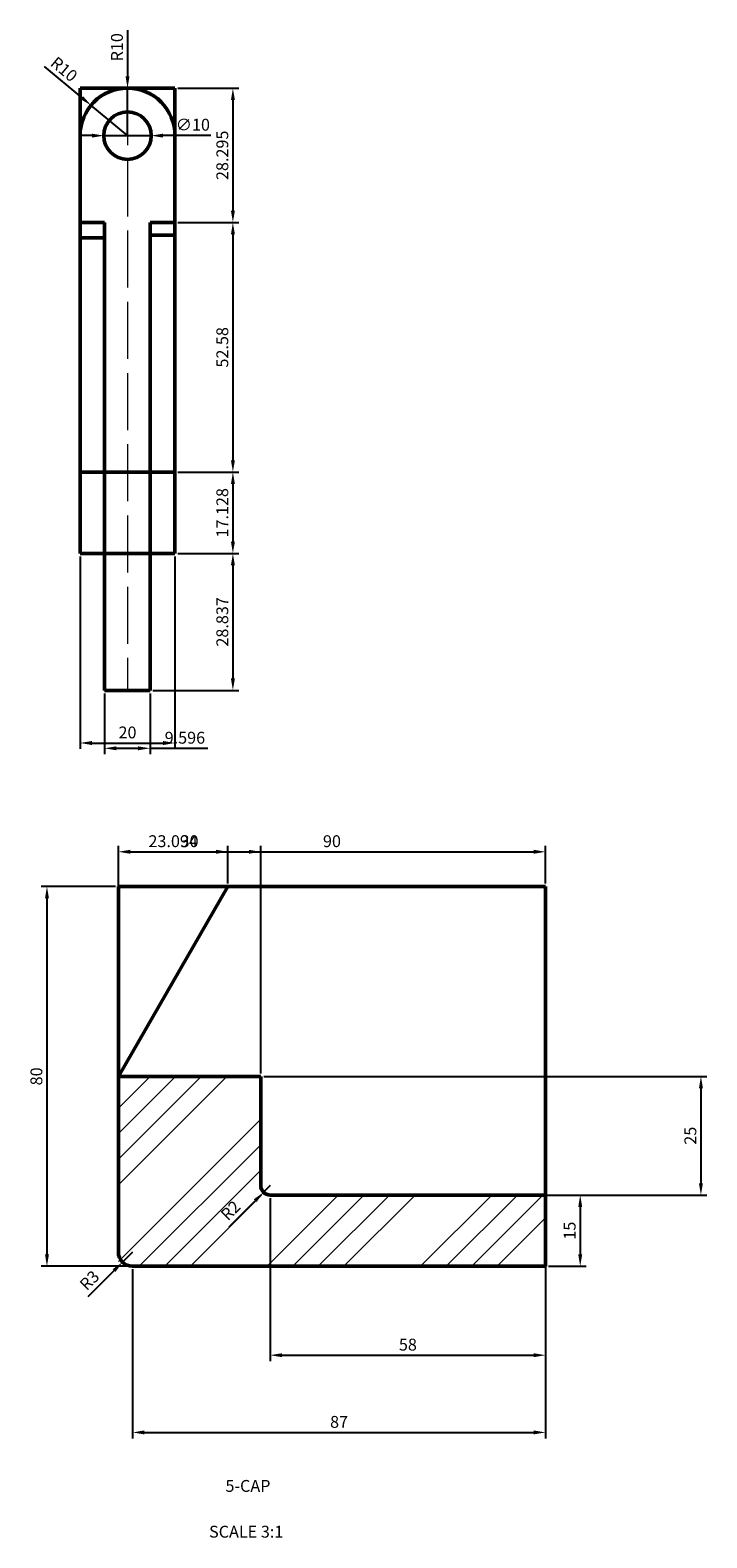
# Model space of a CAD drawing. Units: millimetres. Extents: x 1139 to 1488, y 1435 to 1756.
# Tile 3 of 3: x 1345 to 1488, y 1435 to 1753. Entities that reach past the tile are written whole.
import ezdxf

# ---------------------------------------------------------------- set-up
doc = ezdxf.new("R2010")
doc.units = ezdxf.units.MM
doc.linetypes.add('ACAD_ISO02W100', pattern=[15, 12, -3])
for name, color, linetype, lineweight in [('M-CNTR', 4, 'ACAD_ISO02W100', 18), ('M-DIMS', 2, 'Continuous', 25), ('M-HATC', 8, 'Continuous', 18), ('M-OUTL', 7, 'Continuous', 50), ('M-TEXT', 7, 'Continuous', 25)]:
    doc.layers.add(name, color=color, linetype=linetype, lineweight=lineweight)
doc.styles.get("Standard").update_dxf_attribs({"font": 'arial.ttf'})
doc.dimstyles.new('ISO-25', dxfattribs={"dimtxt": 2.5, "dimasz": 2.5, "dimexe": 1.25, "dimexo": 0.625, "dimtad": 1, "dimtxsty": 'Standard', "dimcen": 2.5, "dimadec": 0, "dimazin": 0, "dimtfac": 1, "dimtmove": 0, "dimatfit": 3, "dimfxl": 1, "dimarcsym": 0})

# ---------------------------------------------------------------- blocks, each defined once
blk = doc.blocks.new('*D22')
at = {"layer": 'Defpoints', "color": 0, "transparency": 16777216}
for p in [(1355.99, 1642.51), (1375.99, 1642.51), (1375.99, 1602.59)]:
    blk.add_point(p, dxfattribs=at)
at = {"layer": 'M-DIMS', "color": 0, "lineweight": -2, "transparency": 16777216}
for p, q in [((1355.99, 1641.89), (1355.99, 1601.34)), ((1375.99, 1641.89), (1375.99, 1601.34)), ((1358.49, 1602.59), (1373.49, 1602.59))]:
    blk.add_line(p, q, dxfattribs=at)
at = {"layer": 'M-DIMS', "color": 0, "transparency": 16777216}
for points in [[(1358.49, 1603.01), (1358.49, 1602.17), (1355.99, 1602.59)], [(1373.49, 1603.01), (1373.49, 1602.17), (1375.99, 1602.59)]]:
    blk.add_solid(points, dxfattribs=at)
at = {"layer": 'M-DIMS', "color": 0, "transparency": 16777216, "insert": (1365.99, 1604.49), "char_height": 2.5, "attachment_point": 5}
blk.add_mtext('20', dxfattribs=at)
blk = doc.blocks.new('*D23')
at = {"layer": 'Defpoints', "color": 0, "transparency": 16777216}
for p in [(1358.3, 1736.9), (1365.99, 1730.51)]:
    blk.add_point(p, dxfattribs=at)
at = {"layer": 'M-DIMS', "color": 0, "lineweight": -2, "transparency": 16777216}
for p, q in [((1348.43, 1745.09), (1356.38, 1738.5)), ((1365.99, 1730.51), (1358.3, 1736.9))]:
    blk.add_line(p, q, dxfattribs=at)
at = {"layer": 'M-DIMS', "color": 0, "transparency": 16777216}
blk.add_solid([(1356.64, 1738.82), (1356.11, 1738.18), (1358.3, 1736.9)], dxfattribs=at)
at = {"layer": 'M-DIMS', "color": 0, "transparency": 16777216, "insert": (1352.42, 1744.25), "char_height": 2.5, "attachment_point": 5, "rotation": 320.2997}
blk.add_mtext('R10', dxfattribs=at)
blk = doc.blocks.new('*D24')
at = {"layer": 'Defpoints', "color": 0, "transparency": 16777216}
for p in [(1394.06, 1532.38), (1396.06, 1507.38), (1486.79, 1507.38)]:
    blk.add_point(p, dxfattribs=at)
at = {"layer": 'M-DIMS', "color": 0, "lineweight": -2, "transparency": 16777216}
for p, q in [((1394.69, 1532.38), (1488.04, 1532.38)), ((1486.79, 1529.88), (1486.79, 1509.88)), ((1396.69, 1507.38), (1488.04, 1507.38))]:
    blk.add_line(p, q, dxfattribs=at)
at = {"layer": 'M-DIMS', "color": 0, "transparency": 16777216}
for points in [[(1486.37, 1529.88), (1487.21, 1529.88), (1486.79, 1532.38)], [(1486.37, 1509.88), (1487.21, 1509.88), (1486.79, 1507.38)]]:
    blk.add_solid(points, dxfattribs=at)
at = {"layer": 'M-DIMS', "color": 0, "transparency": 16777216, "insert": (1484.89, 1519.88), "char_height": 2.5, "attachment_point": 5, "rotation": 90}
blk.add_mtext('25', dxfattribs=at)
blk = doc.blocks.new('*D25')
at = {"layer": 'Defpoints', "color": 0, "transparency": 16777216}
for p in [(1367.06, 1492.38), (1454.06, 1492.38), (1454.06, 1457.39)]:
    blk.add_point(p, dxfattribs=at)
at = {"layer": 'M-DIMS', "color": 0, "lineweight": -2, "transparency": 16777216}
for p, q in [((1367.06, 1491.76), (1367.06, 1456.14)), ((1454.06, 1491.76), (1454.06, 1456.14)), ((1369.56, 1457.39), (1451.56, 1457.39))]:
    blk.add_line(p, q, dxfattribs=at)
at = {"layer": 'M-DIMS', "color": 0, "transparency": 16777216}
for points in [[(1369.56, 1457.81), (1369.56, 1456.98), (1367.06, 1457.39)], [(1451.56, 1457.81), (1451.56, 1456.98), (1454.06, 1457.39)]]:
    blk.add_solid(points, dxfattribs=at)
at = {"layer": 'M-DIMS', "color": 0, "transparency": 16777216, "insert": (1410.56, 1459.29), "char_height": 2.5, "attachment_point": 5}
blk.add_mtext('87', dxfattribs=at)
blk = doc.blocks.new('*D26')
at = {"layer": 'Defpoints', "color": 0, "transparency": 16777216}
for p in [(1396.06, 1507.38), (1454.06, 1507.38), (1454.06, 1473.66)]:
    blk.add_point(p, dxfattribs=at)
at = {"layer": 'M-DIMS', "color": 0, "lineweight": -2, "transparency": 16777216}
for p, q in [((1396.06, 1506.76), (1396.06, 1472.41)), ((1454.06, 1506.76), (1454.06, 1472.41)), ((1398.56, 1473.66), (1451.56, 1473.66))]:
    blk.add_line(p, q, dxfattribs=at)
at = {"layer": 'M-DIMS', "color": 0, "transparency": 16777216}
for points in [[(1398.56, 1474.07), (1398.56, 1473.24), (1396.06, 1473.66)], [(1451.56, 1474.07), (1451.56, 1473.24), (1454.06, 1473.66)]]:
    blk.add_solid(points, dxfattribs=at)
at = {"layer": 'M-DIMS', "color": 0, "transparency": 16777216, "insert": (1425.06, 1475.56), "char_height": 2.5, "attachment_point": 5}
blk.add_mtext('58', dxfattribs=at)
blk = doc.blocks.new('*D27')
at = {"layer": 'Defpoints', "color": 0, "transparency": 16777216}
for p in [(1364.06, 1572.38), (1349.02, 1492.38), (1367.06, 1492.38)]:
    blk.add_point(p, dxfattribs=at)
at = {"layer": 'M-DIMS', "color": 0, "lineweight": -2, "transparency": 16777216}
for p, q in [((1363.44, 1572.38), (1347.77, 1572.38)), ((1349.02, 1569.88), (1349.02, 1494.88)), ((1366.44, 1492.38), (1347.77, 1492.38))]:
    blk.add_line(p, q, dxfattribs=at)
at = {"layer": 'M-DIMS', "color": 0, "transparency": 16777216}
for points in [[(1348.61, 1569.88), (1349.44, 1569.88), (1349.02, 1572.38)], [(1348.61, 1494.88), (1349.44, 1494.88), (1349.02, 1492.38)]]:
    blk.add_solid(points, dxfattribs=at)
at = {"layer": 'M-DIMS', "color": 0, "transparency": 16777216, "insert": (1347.12, 1532.38), "char_height": 2.5, "attachment_point": 5, "rotation": 90}
blk.add_mtext('80', dxfattribs=at)
blk = doc.blocks.new('*D35')
at = {"layer": 'Defpoints', "color": 0, "transparency": 16777216}
for p in [(1375.99, 1740.51), (1375.99, 1712.22), (1388.19, 1712.22)]:
    blk.add_point(p, dxfattribs=at)
at = {"layer": 'M-DIMS', "color": 0, "lineweight": -2, "transparency": 16777216}
for p, q in [((1376.62, 1740.51), (1389.44, 1740.51)), ((1388.19, 1738.01), (1388.19, 1714.72)), ((1376.62, 1712.22), (1389.44, 1712.22))]:
    blk.add_line(p, q, dxfattribs=at)
at = {"layer": 'M-DIMS', "color": 0, "transparency": 16777216}
for points in [[(1387.78, 1738.01), (1388.61, 1738.01), (1388.19, 1740.51)], [(1387.78, 1714.72), (1388.61, 1714.72), (1388.19, 1712.22)]]:
    blk.add_solid(points, dxfattribs=at)
at = {"layer": 'M-DIMS', "color": 0, "transparency": 16777216, "insert": (1386.29, 1726.37), "char_height": 2.5, "attachment_point": 5, "rotation": 90}
blk.add_mtext('28.295', dxfattribs=at)
blk = doc.blocks.new('*D36')
at = {"layer": 'Defpoints', "color": 0, "transparency": 16777216}
for p in [(1375.99, 1712.22), (1375.99, 1659.64), (1388.19, 1659.64)]:
    blk.add_point(p, dxfattribs=at)
at = {"layer": 'M-DIMS', "color": 0, "lineweight": -2, "transparency": 16777216}
for p, q in [((1376.62, 1712.22), (1389.44, 1712.22)), ((1388.19, 1709.72), (1388.19, 1662.14)), ((1376.62, 1659.64), (1389.44, 1659.64))]:
    blk.add_line(p, q, dxfattribs=at)
at = {"layer": 'M-DIMS', "color": 0, "transparency": 16777216}
for points in [[(1387.78, 1709.72), (1388.61, 1709.72), (1388.19, 1712.22)], [(1387.78, 1662.14), (1388.61, 1662.14), (1388.19, 1659.64)]]:
    blk.add_solid(points, dxfattribs=at)
at = {"layer": 'M-DIMS', "color": 0, "transparency": 16777216, "insert": (1386.29, 1685.93), "char_height": 2.5, "attachment_point": 5, "rotation": 90}
blk.add_mtext('52.58', dxfattribs=at)
blk = doc.blocks.new('*D37')
at = {"layer": 'Defpoints', "color": 0, "transparency": 16777216}
for p in [(1375.99, 1659.64), (1375.99, 1642.51), (1388.19, 1642.51)]:
    blk.add_point(p, dxfattribs=at)
at = {"layer": 'M-DIMS', "color": 0, "lineweight": -2, "transparency": 16777216}
for p, q in [((1376.62, 1659.64), (1389.44, 1659.64)), ((1388.19, 1657.14), (1388.19, 1645.01)), ((1376.62, 1642.51), (1389.44, 1642.51))]:
    blk.add_line(p, q, dxfattribs=at)
at = {"layer": 'M-DIMS', "color": 0, "transparency": 16777216}
for points in [[(1387.78, 1657.14), (1388.61, 1657.14), (1388.19, 1659.64)], [(1387.78, 1645.01), (1388.61, 1645.01), (1388.19, 1642.51)]]:
    blk.add_solid(points, dxfattribs=at)
at = {"layer": 'M-DIMS', "color": 0, "transparency": 16777216, "insert": (1386.29, 1651.08), "char_height": 2.5, "attachment_point": 5, "rotation": 90}
blk.add_mtext('17.128', dxfattribs=at)
blk = doc.blocks.new('*D38')
at = {"layer": 'Defpoints', "color": 0, "transparency": 16777216}
for p in [(1375.99, 1642.51), (1370.73, 1613.68), (1388.19, 1613.68)]:
    blk.add_point(p, dxfattribs=at)
at = {"layer": 'M-DIMS', "color": 0, "lineweight": -2, "transparency": 16777216}
for p, q in [((1376.62, 1642.51), (1389.44, 1642.51)), ((1388.19, 1640.01), (1388.19, 1616.18)), ((1371.36, 1613.68), (1389.44, 1613.68))]:
    blk.add_line(p, q, dxfattribs=at)
at = {"layer": 'M-DIMS', "color": 0, "transparency": 16777216}
for points in [[(1387.78, 1640.01), (1388.61, 1640.01), (1388.19, 1642.51)], [(1387.78, 1616.18), (1388.61, 1616.18), (1388.19, 1613.68)]]:
    blk.add_solid(points, dxfattribs=at)
at = {"layer": 'M-DIMS', "color": 0, "transparency": 16777216, "insert": (1386.29, 1628.1), "char_height": 2.5, "attachment_point": 5, "rotation": 90}
blk.add_mtext('28.837', dxfattribs=at)
blk = doc.blocks.new('*D39')
at = {"layer": 'Defpoints', "color": 0, "transparency": 16777216}
for p in [(1361.14, 1613.68), (1370.73, 1613.68), (1370.73, 1601.48)]:
    blk.add_point(p, dxfattribs=at)
at = {"layer": 'M-DIMS', "color": 0, "lineweight": -2, "transparency": 16777216}
for p, q in [((1361.14, 1613.05), (1361.14, 1600.23)), ((1370.73, 1613.05), (1370.73, 1600.23)), ((1363.64, 1601.48), (1368.23, 1601.48)), ((1370.73, 1601.48), (1382.92, 1601.48))]:
    blk.add_line(p, q, dxfattribs=at)
at = {"layer": 'M-DIMS', "color": 0, "transparency": 16777216}
for points in [[(1363.64, 1601.89), (1363.64, 1601.06), (1361.14, 1601.48)], [(1368.23, 1601.89), (1368.23, 1601.06), (1370.73, 1601.48)]]:
    blk.add_solid(points, dxfattribs=at)
at = {"layer": 'M-DIMS', "color": 0, "transparency": 16777216, "insert": (1378.08, 1603.38), "char_height": 2.5, "attachment_point": 5}
blk.add_mtext('9.596', dxfattribs=at)
blk = doc.blocks.new('*D47')
at = {"layer": 'Defpoints', "color": 0, "transparency": 16777216}
for p in [(1454.06, 1579.68), (1364.06, 1572.38), (1454.06, 1572.38)]:
    blk.add_point(p, dxfattribs=at)
at = {"layer": 'M-DIMS', "color": 0, "lineweight": -2, "transparency": 16777216}
for p, q in [((1364.06, 1573.01), (1364.06, 1580.93)), ((1366.56, 1579.68), (1451.56, 1579.68)), ((1454.06, 1573.01), (1454.06, 1580.93))]:
    blk.add_line(p, q, dxfattribs=at)
at = {"layer": 'M-DIMS', "color": 0, "transparency": 16777216}
for points in [[(1366.56, 1580.1), (1366.56, 1579.27), (1364.06, 1579.68)], [(1451.56, 1580.1), (1451.56, 1579.27), (1454.06, 1579.68)]]:
    blk.add_solid(points, dxfattribs=at)
at = {"layer": 'M-DIMS', "color": 0, "transparency": 16777216, "insert": (1409.06, 1581.59), "char_height": 2.5, "attachment_point": 5}
blk.add_mtext('90', dxfattribs=at)
blk = doc.blocks.new('*D48')
at = {"layer": 'Defpoints', "color": 0, "transparency": 16777216}
for p in [(1387.16, 1579.68), (1364.06, 1572.38), (1387.16, 1572.38)]:
    blk.add_point(p, dxfattribs=at)
at = {"layer": 'M-DIMS', "color": 0, "lineweight": -2, "transparency": 16777216}
for p, q in [((1364.06, 1573.01), (1364.06, 1580.93)), ((1366.56, 1579.68), (1384.66, 1579.68)), ((1387.16, 1573.01), (1387.16, 1580.93))]:
    blk.add_line(p, q, dxfattribs=at)
at = {"layer": 'M-DIMS', "color": 0, "transparency": 16777216}
for points in [[(1366.56, 1580.1), (1366.56, 1579.27), (1364.06, 1579.68)], [(1384.66, 1580.1), (1384.66, 1579.27), (1387.16, 1579.68)]]:
    blk.add_solid(points, dxfattribs=at)
at = {"layer": 'M-DIMS', "color": 0, "transparency": 16777216, "insert": (1375.61, 1581.59), "char_height": 2.5, "attachment_point": 5}
blk.add_mtext('23.094', dxfattribs=at)
blk = doc.blocks.new('*D49')
at = {"layer": 'Defpoints', "color": 0, "transparency": 16777216}
for p in [(1394.06, 1579.68), (1364.06, 1532.38), (1394.06, 1532.38)]:
    blk.add_point(p, dxfattribs=at)
at = {"layer": 'M-DIMS', "color": 0, "lineweight": -2, "transparency": 16777216}
for p, q in [((1364.06, 1533.01), (1364.06, 1580.93)), ((1366.56, 1579.68), (1391.56, 1579.68)), ((1394.06, 1533.01), (1394.06, 1580.93))]:
    blk.add_line(p, q, dxfattribs=at)
at = {"layer": 'M-DIMS', "color": 0, "transparency": 16777216}
for points in [[(1366.56, 1580.1), (1366.56, 1579.27), (1364.06, 1579.68)], [(1391.56, 1580.1), (1391.56, 1579.27), (1394.06, 1579.68)]]:
    blk.add_solid(points, dxfattribs=at)
at = {"layer": 'M-DIMS', "color": 0, "transparency": 16777216, "insert": (1379.06, 1581.59), "char_height": 2.5, "attachment_point": 5}
blk.add_mtext('30', dxfattribs=at)
blk = doc.blocks.new('*D50')
at = {"layer": 'Defpoints', "color": 0, "transparency": 16777216}
for p in [(1454.06, 1507.38), (1454.06, 1492.38), (1461.36, 1492.38)]:
    blk.add_point(p, dxfattribs=at)
at = {"layer": 'M-DIMS', "color": 0, "lineweight": -2, "transparency": 16777216}
for p, q in [((1454.69, 1507.38), (1462.61, 1507.38)), ((1461.36, 1504.88), (1461.36, 1494.88)), ((1454.69, 1492.38), (1462.61, 1492.38))]:
    blk.add_line(p, q, dxfattribs=at)
at = {"layer": 'M-DIMS', "color": 0, "transparency": 16777216}
for points in [[(1460.95, 1504.88), (1461.78, 1504.88), (1461.36, 1507.38)], [(1460.95, 1494.88), (1461.78, 1494.88), (1461.36, 1492.38)]]:
    blk.add_solid(points, dxfattribs=at)
at = {"layer": 'M-DIMS', "color": 0, "transparency": 16777216, "insert": (1459.46, 1499.88), "char_height": 2.5, "attachment_point": 5, "rotation": 90}
blk.add_mtext('15', dxfattribs=at)
blk = doc.blocks.new('*D54')
at = {"layer": 'Defpoints', "color": 0, "transparency": 16777216}
for p in [(1365.99, 1740.51), (1365.99, 1730.51)]:
    blk.add_point(p, dxfattribs=at)
at = {"layer": 'M-DIMS', "color": 0, "lineweight": -2, "transparency": 16777216}
for p, q in [((1365.99, 1752.73), (1365.99, 1743.01)), ((1365.99, 1730.51), (1365.99, 1740.51))]:
    blk.add_line(p, q, dxfattribs=at)
at = {"layer": 'M-DIMS', "color": 0, "transparency": 16777216}
blk.add_solid([(1365.58, 1743.01), (1366.41, 1743.01), (1365.99, 1740.51)], dxfattribs=at)
at = {"layer": 'M-DIMS', "color": 0, "transparency": 16777216, "insert": (1364.09, 1749.12), "char_height": 2.5, "attachment_point": 5, "rotation": 89.9981}
blk.add_mtext('R10', dxfattribs=at)
blk = doc.blocks.new('*D55')
at = {"layer": 'Defpoints', "color": 0, "transparency": 16777216}
for p in [(1360.99, 1730.51), (1370.99, 1730.51)]:
    blk.add_point(p, dxfattribs=at)
at = {"layer": 'M-DIMS', "color": 0, "lineweight": -2, "transparency": 16777216}
for p, q in [((1358.49, 1730.51), (1355.99, 1730.51)), ((1360.99, 1730.51), (1370.99, 1730.51)), ((1383.54, 1730.51), (1373.49, 1730.51))]:
    blk.add_line(p, q, dxfattribs=at)
at = {"layer": 'M-DIMS', "color": 0, "transparency": 16777216}
for points in [[(1358.49, 1730.93), (1358.49, 1730.1), (1360.99, 1730.51)], [(1373.49, 1730.93), (1373.49, 1730.1), (1370.99, 1730.51)]]:
    blk.add_solid(points, dxfattribs=at)
at = {"layer": 'M-DIMS', "color": 0, "transparency": 16777216, "insert": (1379.76, 1732.49), "char_height": 2.5, "attachment_point": 5, "rotation": 0.0002}
blk.add_mtext('∅10', dxfattribs=at)
blk = doc.blocks.new('*D56')
at = {"layer": 'Defpoints', "color": 0, "transparency": 16777216}
for p in [(1364.94, 1493.26), (1367.06, 1495.38)]:
    blk.add_point(p, dxfattribs=at)
at = {"layer": 'M-DIMS', "color": 0, "lineweight": -2, "transparency": 16777216}
for p, q in [((1367.06, 1495.38), (1364.94, 1493.26)), ((1357.67, 1485.99), (1363.18, 1491.49))]:
    blk.add_line(p, q, dxfattribs=at)
at = {"layer": 'M-DIMS', "color": 0, "transparency": 16777216}
blk.add_solid([(1362.88, 1491.79), (1363.47, 1491.2), (1364.94, 1493.26)], dxfattribs=at)
at = {"layer": 'M-DIMS', "color": 0, "transparency": 16777216, "insert": (1358.2, 1489.2), "char_height": 2.5, "attachment_point": 5, "rotation": 45.0101}
blk.add_mtext('R3', dxfattribs=at)
blk = doc.blocks.new('*D57')
at = {"layer": 'Defpoints', "color": 0, "transparency": 16777216}
for p in [(1396.06, 1509.38), (1394.65, 1507.97)]:
    blk.add_point(p, dxfattribs=at)
at = {"layer": 'M-DIMS', "color": 0, "lineweight": -2, "transparency": 16777216}
for p, q in [((1396.06, 1509.38), (1394.65, 1507.97)), ((1387.4, 1500.72), (1392.88, 1506.2))]:
    blk.add_line(p, q, dxfattribs=at)
at = {"layer": 'M-DIMS', "color": 0, "transparency": 16777216}
blk.add_solid([(1392.59, 1506.5), (1393.18, 1505.91), (1394.65, 1507.97)], dxfattribs=at)
at = {"layer": 'M-DIMS', "color": 0, "transparency": 16777216, "insert": (1387.93, 1503.91), "char_height": 2.5, "attachment_point": 5, "rotation": 44.9949}
blk.add_mtext('R2', dxfattribs=at)

msp = doc.modelspace()

# ---------------------------------------------------------------- hatches: boundary and pattern name
at = {"layer": 'M-HATC'}
h = msp.add_hatch(dxfattribs=at)
h.set_pattern_fill('ANSI34', color=256, scale=1.2)
h.paths.add_polyline_path([(1394.0639, 1532.3836), (1364.0639, 1532.3836), (1364.0639, 1492.3836), (1454.0639, 1492.3836), (1454.0639, 1507.3836), (1394.0639, 1507.3836)])

# ---------------------------------------------------------------- linework, layer by layer
at = {"layer": 'M-CNTR'}
msp.add_line((1365.9927, 1740.514), (1365.9927, 1613.6771), dxfattribs=at)
at = {"layer": 'M-OUTL'}
for p, q in [((1355.9927, 1740.514), (1375.9927, 1740.514)), ((1355.9927, 1642.514), (1355.9927, 1740.514)), ((1375.9927, 1740.514), (1375.9927, 1642.514)), ((1361.1384, 1712.2186), (1355.9927, 1712.2186)), ((1361.1384, 1712.2186), (1361.1384, 1613.6771)), ((1370.7347, 1712.2186), (1370.7347, 1613.6771)), ((1370.7347, 1712.2186), (1375.9927, 1712.2186)), ((1361.1384, 1709.0208), (1355.9927, 1709.0208)), ((1370.7347, 1709.567), (1375.9927, 1709.567)), ((1355.9927, 1659.6415), (1375.9927, 1659.6415)), ((1375.9927, 1642.514), (1355.9927, 1642.514)), ((1361.1384, 1613.6771), (1370.7347, 1613.6771)), ((1364.0639, 1572.3836), (1364.0639, 1495.3836)), ((1364.0639, 1532.3836), (1387.1579, 1572.3836)), ((1364.0639, 1572.3836), (1387.1579, 1572.3836)), ((1387.1579, 1572.3836), (1454.0639, 1572.3836)), ((1454.0639, 1507.3836), (1454.0639, 1572.3836)), ((1364.0639, 1532.3836), (1394.0639, 1532.3836)), ((1394.0639, 1509.3836), (1394.0639, 1532.3836)), ((1454.0639, 1507.3836), (1396.0639, 1507.3836)), ((1454.0639, 1492.3836), (1454.0639, 1507.3836)), ((1367.0639, 1492.3836), (1454.0639, 1492.3836))]:
    msp.add_line(p, q, dxfattribs=at)
msp.add_circle((1365.9927, 1730.514), 5, dxfattribs=at)
for centre, radius, start, end in [((1365.9927, 1730.514), 10, 0, 180), ((1396.0639, 1509.3836), 2, 180, 270), ((1367.0639, 1495.3836), 3, 180, 270)]:
    msp.add_arc(centre, radius, start, end, dxfattribs=at)

# ---------------------------------------------------------------- texts
at = {"layer": 'M-TEXT', "char_height": 2.5, "attachment_point": 1}
for s, width, insert in [('5-CAP', 40.100497, (1386.6244, 1447.3761)), ('SCALE 3:1', 36.422799, (1383.1725, 1437.7335))]:
    msp.add_mtext_dynamic_manual_height_columns(s, width=width, gutter_width=12.5, heights=[0], dxfattribs=dict(at, insert=insert))

# ---------------------------------------------------------------- dimensions: what is measured, and where the dimension line sits
at = {"layer": 'M-DIMS'}
for center, mpoint, picture, middle in [((1365.9927, 1730.514), (1365.993, 1740.514), '*D54', (1364.0919, 1749.1217)), ((1396.0639, 1509.3836), (1394.6495, 1507.9695), '*D57', (1387.926, 1503.9058)), ((1367.0639, 1495.3836), (1364.9429, 1493.2619), '*D56', (1358.1957, 1489.2031))]:
    dim = msp.add_radius_dim(center=center, mpoint=mpoint, dimstyle='ISO-25', override={"dimdec": 0, "dimlfac": 1, "dimrnd": 0, "dimzin": 0, "dimdsep": 46, "dimlunit": 2}, dxfattribs=at)
    dim.commit()
    dim.dimension.update_dxf_attribs({"geometry": picture, "text_midpoint": middle})
dim = msp.add_radius_dim(center=(1365.9927, 1730.514), mpoint=(1358.2987, 1736.9017), dimstyle='ISO-25', override={"dimclrd": 0, "dimclre": 0, "dimclrt": 0}, dxfattribs=at)
dim.commit()
dim.dimension.update_dxf_attribs({"geometry": '*D23', "text_midpoint": (1351.2064, 1742.7899), "dimtype": 164})
for base, p1, p2, override, picture, middle in [((1388.1927, 1712.2186), (1375.9927, 1740.514), (1375.9927, 1712.2186), {"dimdec": 3, "dimlfac": 1, "dimrnd": 0, "dimzin": 0, "dimdsep": 46, "dimlunit": 2}, '*D35', (1386.2912, 1726.3663)), ((1388.1927, 1659.6415), (1375.9927, 1712.2186), (1375.9927, 1659.6415), {"dimdec": 2, "dimlfac": 1, "dimrnd": 0, "dimzin": 0, "dimdsep": 46, "dimlunit": 2}, '*D36', (1386.2912, 1685.93)), ((1388.19267, 1642.51398), (1375.99267, 1659.64153), (1375.99267, 1642.51398), {"dimdec": 3, "dimlfac": 1, "dimrnd": 0, "dimzin": 0, "dimdsep": 46, "dimlunit": 2}, '*D37', (1386.29124, 1651.07776)), ((1388.1927, 1613.6771), (1375.9927, 1642.514), (1370.7347, 1613.6771), {"dimdec": 3, "dimlfac": 1, "dimrnd": 0, "dimzin": 0, "dimdsep": 46, "dimlunit": 2}, '*D38', (1386.2904, 1628.0955)), ((1349.0227, 1492.3836), (1364.0639, 1572.3836), (1367.0639, 1492.3836), {"dimclrd": 0, "dimclre": 0, "dimclrt": 0}, '*D27', (1347.1212, 1532.3836)), ((1486.7887, 1507.3836), (1394.0639, 1532.3836), (1396.0639, 1507.3836), {"dimclrd": 0, "dimclre": 0, "dimclrt": 0}, '*D24', (1484.8873, 1519.8836)), ((1461.3639, 1492.3836), (1454.0639, 1507.3836), (1454.0639, 1492.3836), {"dimdec": 0, "dimlfac": 1, "dimrnd": 0, "dimzin": 0, "dimdsep": 46, "dimlunit": 2}, '*D50', (1459.4624, 1499.8836))]:
    dim = msp.add_linear_dim(base=base, p1=p1, p2=p2, angle=90, dimstyle='ISO-25', override=override, dxfattribs=at)
    dim.commit()
    dim.dimension.update_dxf_attribs({"geometry": picture, "text_midpoint": middle})
dim = msp.add_diameter_dim_2p(p1=(1360.9927, 1730.514), p2=(1370.9927, 1730.514), dimstyle='ISO-25', override={"dimdec": 0, "dimlfac": 1, "dimrnd": 0, "dimzin": 0, "dimdsep": 46, "dimlunit": 2}, dxfattribs=at)
dim.commit()
dim.dimension.update_dxf_attribs({"geometry": '*D55', "text_midpoint": (1379.764, 1730.514)})
for base, p1, p2, override, picture, middle in [((1375.9927, 1602.5909), (1355.9927, 1642.514), (1375.9927, 1642.514), {"dimclrd": 0, "dimclre": 0, "dimclrt": 0}, '*D22', (1365.9927, 1604.4923)), ((1370.7347, 1601.4771), (1361.1384, 1613.6771), (1370.7347, 1613.6771), {"dimdec": 3, "dimlfac": 1, "dimrnd": 0, "dimzin": 0, "dimdsep": 46, "dimlunit": 2}, '*D39', (1378.077, 1603.3785)), ((1387.1579, 1579.6836), (1364.0639, 1572.3836), (1387.1579, 1572.3836), {"dimdec": 3, "dimlfac": 1, "dimrnd": 0, "dimzin": 0, "dimdsep": 46, "dimlunit": 2}, '*D48', (1375.6109, 1581.5859)), ((1394.0639, 1579.6836), (1364.0639, 1532.3836), (1394.0639, 1532.3836), {"dimdec": 0, "dimlfac": 1, "dimrnd": 0, "dimzin": 0, "dimdsep": 46, "dimlunit": 2}, '*D49', (1379.0639, 1581.5859)), ((1454.0639, 1579.6836), (1364.0639, 1572.3836), (1454.0639, 1572.3836), {"dimdec": 0, "dimlfac": 1, "dimrnd": 0, "dimzin": 0, "dimdsep": 46, "dimlunit": 2}, '*D47', (1409.0639, 1581.585)), ((1454.0639, 1473.6569), (1396.0639, 1507.3836), (1454.0639, 1507.3836), {"dimclrd": 0, "dimclre": 0, "dimclrt": 0}, '*D26', (1425.0639, 1475.5583)), ((1454.0639, 1457.3924), (1367.0639, 1492.3836), (1454.0639, 1492.3836), {"dimclrd": 0, "dimclre": 0, "dimclrt": 0}, '*D25', (1410.5639, 1459.2938))]:
    dim = msp.add_linear_dim(base=base, p1=p1, p2=p2, dimstyle='ISO-25', override=override, dxfattribs=at)
    dim.commit()
    dim.dimension.update_dxf_attribs({"geometry": picture, "text_midpoint": middle})

doc.saveas('drawing.dxf')
